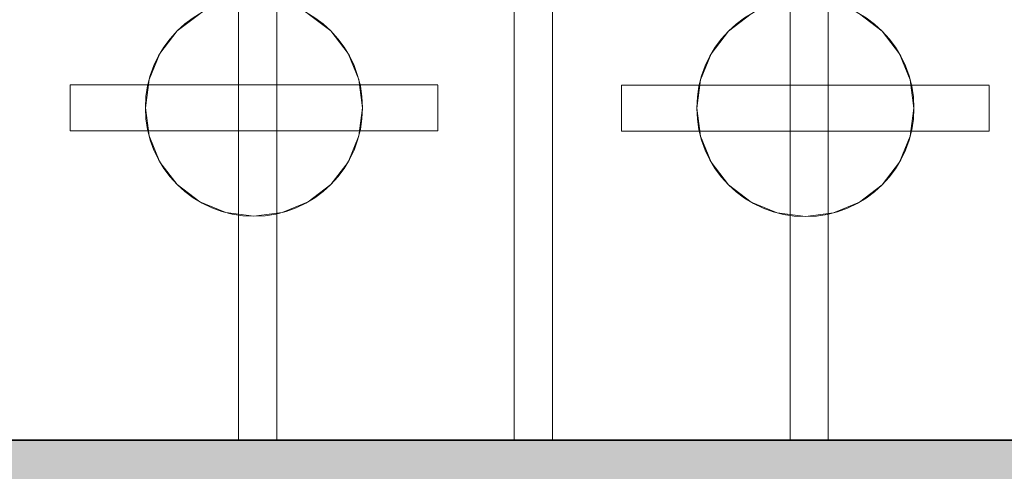
# Model space of a CAD drawing. Units: inches. Extents: x 2696 to 3240, y 1564 to 2310.
# Tile 69 of 76: x 3144.264 to 3152.299, y 2074.447 to 2078.132. Entities that reach past the tile are written whole.
import ezdxf

# ---------------------------------------------------------------- set-up
doc = ezdxf.new("R2010")
doc.units = ezdxf.units.IN
for name, color, linetype, lineweight in [('A-ANNO-DIMS', 3, 'Continuous', 18), ('A-FLOR-FIXT', 8, 'Continuous', 18), ('A-FURN', 251, 'Continuous', 13), ('A-WALL', 7, 'Continuous', 35), ('A-WALL-PATT', 9, 'Continuous', 13)]:
    doc.layers.add(name, color=color, linetype=linetype, lineweight=lineweight)
doc.layers.add('FURNITURE', color=250, linetype='Continuous')
doc.styles.add('TIMES NEW', font='times.ttf')
doc.dimstyles.new('Siddhuu', dxfattribs={"dimtxt": 6, "dimasz": 2.5, "dimexe": 1.25, "dimexo": 0.625, "dimtad": 1, "dimdec": 1, "dimlunit": 4, "dimtxsty": 'TIMES NEW', "dimcen": 2.5, "dimclrd": 256, "dimclre": 1, "dimclrt": 7, "dimadec": 0, "dimazin": 0, "dimtfac": 1, "dimtdec": 1, "dimtmove": 0, "dimatfit": 3, "dimfxl": 1, "dimtolj": 1, "dimlwd": -1, "dimarcsym": 0})

# ---------------------------------------------------------------- blocks, each defined once
blk = doc.blocks.new('A$C1af1f523')
at = {"layer": 'A-FURN'}
for p, q in [((-2.9003, 3.9351), (-2.9003, 0.9365)), ((-2.9003, 3.9351, 0.5), (-2.9003, 0.9365, 0.5)), ((-2.9003, 3.9351), (-2.9003, 3.9351, 0.5)), ((-2.5253, 3.9351), (-2.9003, 3.9351)), ((-2.5253, 3.9351, 0.5), (-2.9003, 3.9351, 0.5)), ((-2.5253, 3.9351), (-2.5253, 0.9365)), ((-2.5253, 3.9351, 0.5), (-2.5253, 0.9365, 0.5)), ((-2.5253, 3.9351), (-2.5253, 3.9351, 0.5)), ((-2.7128, 3.3215), (-2.7128, 3.3215, 0.5)), ((-2.9421, 3.2913), (-2.9421, 3.2913, 0.5)), ((-2.4835, 3.2913), (-2.4835, 3.2913, 0.5)), ((-3.1558, 3.2028), (-3.1558, 3.2028, 0.5)), ((-2.2698, 3.2028), (-2.2698, 3.2028, 0.5)), ((-3.3393, 3.062), (-3.3393, 3.062, 0.5)), ((-2.0863, 3.062), (-2.0863, 3.062, 0.5)), ((-1.9455, 2.8785), (-1.9455, 2.8785, 0.5)), ((-1.857, 2.6648), (-1.857, 2.6648, 0.5)), ((0, 2.5605), (-4.2116, 2.5605)), ((0, 2.5605, 0.5), (-4.2116, 2.5605, 0.5)), ((-1.8268, 2.4355), (-1.8268, 2.4355, 0.5)), ((0, 2.248), (-4.2116, 2.248)), ((0, 2.248, 0.5), (-4.2116, 2.248, 0.5)), ((-1.857, 2.2061), (-1.857, 2.2061, 0.5)), ((-1.9455, 1.9924), (-1.9455, 1.9924, 0.5)), ((-3.3393, 1.8089), (-3.3393, 1.8089, 0.5)), ((-2.0863, 1.8089), (-2.0863, 1.8089, 0.5)), ((-3.1558, 1.6681), (-3.1558, 1.6681, 0.5)), ((-2.2698, 1.6681), (-2.2698, 1.6681, 0.5)), ((-2.9421, 1.5796), (-2.9421, 1.5796, 0.5)), ((-2.7128, 1.5494), (-2.7128, 1.5494, 0.5)), ((-2.4835, 1.5796), (-2.4835, 1.5796, 0.5)), ((-2.9003, 0.9365), (-2.9003, 0.9365, 0.5)), ((-2.5253, 0.9365), (-2.8979, 0.9365)), ((-2.5253, 0.9365, 0.5), (-2.8979, 0.9365, 0.5)), ((-2.8979, 0.9365), (-2.8979, 0.9365, 0.5)), ((-2.5253, 0.9365), (-2.5253, 0.9365, 0.5)), ((0, 0.3125), (-6.5015, 0.3125)), ((0, 0.3125, 0.5), (-6.5015, 0.3125, 0.5)), ((0, 0), (-6.5015, 0)), ((0, 0, 0.5), (-6.5015, 0, 0.5)), ((-2.898, -0.5642), (-2.898, -3.5628)), ((-2.898, -0.5642, 0.5), (-2.898, -3.5628, 0.5)), ((-2.898, -0.5642), (-2.898, -0.5642, 0.5)), ((-2.523, -0.5642), (-2.898, -0.5642)), ((-2.523, -0.5642, 0.5), (-2.898, -0.5642, 0.5)), ((-2.523, -0.5642), (-2.523, -3.5628)), ((-2.523, -0.5642, 0.5), (-2.523, -3.5628, 0.5)), ((-2.523, -0.5642), (-2.523, -0.5642, 0.5)), ((-2.7105, -1.1778), (-2.7105, -1.1778, 0.5)), ((-2.9398, -1.208), (-2.9398, -1.208, 0.5)), ((-2.4812, -1.208), (-2.4812, -1.208, 0.5)), ((-3.1535, -1.2965), (-3.1535, -1.2965, 0.5)), ((-2.2675, -1.2965), (-2.2675, -1.2965, 0.5)), ((-3.337, -1.4373), (-3.337, -1.4373, 0.5)), ((-2.084, -1.4373), (-2.084, -1.4373, 0.5)), ((-1.9432, -1.6208), (-1.9432, -1.6208, 0.5)), ((-1.8547, -1.8345), (-1.8547, -1.8345, 0.5)), ((0, -1.9388), (-4.2094, -1.9388)), ((0, -1.9388, 0.5), (-4.2094, -1.9388, 0.5)), ((-1.8245, -2.0638), (-1.8245, -2.0638, 0.5)), ((0, -2.2513), (-4.2094, -2.2513)), ((0, -2.2513, 0.5), (-4.2094, -2.2513, 0.5)), ((-1.8547, -2.2931), (-1.8547, -2.2931, 0.5)), ((-1.9432, -2.5068), (-1.9432, -2.5068, 0.5)), ((-3.337, -2.6903), (-3.337, -2.6903, 0.5)), ((-2.084, -2.6903), (-2.084, -2.6903, 0.5)), ((-3.1535, -2.8311), (-3.1535, -2.8311, 0.5)), ((-2.2675, -2.8311), (-2.2675, -2.8311, 0.5)), ((-2.9398, -2.9196), (-2.9398, -2.9196, 0.5)), ((-2.7105, -2.9498), (-2.7105, -2.9498, 0.5)), ((-2.4812, -2.9196), (-2.4812, -2.9196, 0.5)), ((-2.898, -3.5628), (-2.898, -3.5628, 0.5)), ((-2.523, -3.5628), (-2.8956, -3.5628)), ((-2.523, -3.5628, 0.5), (-2.8956, -3.5628, 0.5)), ((-2.8956, -3.5628), (-2.8956, -3.5628, 0.5)), ((-2.523, -3.5628), (-2.523, -3.5628, 0.5))]:
    blk.add_line(p, q, dxfattribs=at)
for centre in [(-2.7128, 2.4355), (-2.7128, 2.4355, 0.5), (-2.7105, -2.0638), (-2.7105, -2.0638, 0.5)]:
    blk.add_circle(centre, 0.886, dxfattribs=at)
at = {"layer": 'FURNITURE'}
for p, q in [((0, 2.5605), (0, 2.5605, 0.5)), ((0, 2.248), (0, 2.248, 0.5)), ((0, 0.3125), (0, 0.3125, 0.5)), ((0, 0), (0, 0, 0.5)), ((0, -1.9388), (0, -1.9388, 0.5)), ((0, -2.2513), (0, -2.2513, 0.5))]:
    blk.add_line(p, q, dxfattribs=at)
at = {"layer": 'A-FURN'}
mesh = blk.add_polyface(dxfattribs=at)
corners = [(-2.9003, 0.9365, 0.5), (-2.9003, 3.9351), (-2.9003, 0.9365), (-2.9003, 3.9351, 0.5)]
mesh.append_faces([[corners[k] for k in face] for face in [(2, 1, 0), (3, 0, 1)]], dxfattribs={"vtx1": -1})
mesh = blk.add_polyface(dxfattribs=at)
corners = [(-2.5253, 3.9351, 0.5), (-2.9003, 3.9351), (-2.9003, 3.9351, 0.5), (-2.5253, 3.9351)]
mesh.append_faces([[corners[k] for k in face] for face in [(2, 1, 0), (3, 0, 1)]], dxfattribs={"vtx1": -1})
mesh = blk.add_polyface(dxfattribs=at)
corners = [(-2.5253, 0.9365, 0.5), (-2.5253, 3.9351), (-2.5253, 0.9365), (-2.5253, 3.9351, 0.5)]
mesh.append_faces([[corners[k] for k in face] for face in [(2, 1, 0), (3, 0, 1)]], dxfattribs={"vtx1": -1})
mesh = blk.add_polyface(dxfattribs=at)
corners = [(-2.7128, 3.3215), (-2.9421, 3.2913, 0.5), (-2.9421, 3.2913), (-2.7128, 3.3215, 0.5)]
mesh.append_faces([[corners[k] for k in face] for face in [(2, 1, 0), (3, 0, 1)]], dxfattribs={"vtx1": -1})
mesh = blk.add_polyface(dxfattribs=at)
corners = [(-2.4835, 3.2913), (-2.7128, 3.3215, 0.5), (-2.7128, 3.3215), (-2.4835, 3.2913, 0.5)]
mesh.append_faces([[corners[k] for k in face] for face in [(2, 1, 0), (3, 0, 1)]], dxfattribs={"vtx1": -1})
mesh = blk.add_polyface(dxfattribs=at)
corners = [(-2.9421, 3.2913), (-3.1558, 3.2028, 0.5), (-3.1558, 3.2028), (-2.9421, 3.2913, 0.5)]
mesh.append_faces([[corners[k] for k in face] for face in [(2, 1, 0), (3, 0, 1)]], dxfattribs={"vtx1": -1})
mesh = blk.add_polyface(dxfattribs=at)
corners = [(-2.2698, 3.2028), (-2.4835, 3.2913, 0.5), (-2.4835, 3.2913), (-2.2698, 3.2028, 0.5)]
mesh.append_faces([[corners[k] for k in face] for face in [(2, 1, 0), (3, 0, 1)]], dxfattribs={"vtx1": -1})
mesh = blk.add_polyface(dxfattribs=at)
corners = [(-3.1558, 3.2028), (-3.3393, 3.062, 0.5), (-3.3393, 3.062), (-3.1558, 3.2028, 0.5)]
mesh.append_faces([[corners[k] for k in face] for face in [(2, 1, 0), (3, 0, 1)]], dxfattribs={"vtx1": -1})
mesh = blk.add_polyface(dxfattribs=at)
corners = [(-2.0863, 3.062), (-2.2698, 3.2028, 0.5), (-2.2698, 3.2028), (-2.0863, 3.062, 0.5)]
mesh.append_faces([[corners[k] for k in face] for face in [(2, 1, 0), (3, 0, 1)]], dxfattribs={"vtx1": -1})
mesh = blk.add_polyface(dxfattribs=at)
corners = [(-3.3393, 3.062, 0.5), (-3.4801, 2.8785), (-3.3393, 3.062), (-3.4801, 2.8785, 0.5)]
mesh.append_faces([[corners[k] for k in face] for face in [(2, 1, 0), (3, 0, 1)]], dxfattribs={"vtx1": -1})
mesh = blk.add_polyface(dxfattribs=at)
corners = [(-1.9455, 2.8785, 0.5), (-2.0863, 3.062), (-1.9455, 2.8785), (-2.0863, 3.062, 0.5)]
mesh.append_faces([[corners[k] for k in face] for face in [(2, 1, 0), (3, 0, 1)]], dxfattribs={"vtx1": -1})
mesh = blk.add_polyface(dxfattribs=at)
corners = [(-1.857, 2.6648, 0.5), (-1.9455, 2.8785), (-1.857, 2.6648), (-1.9455, 2.8785, 0.5)]
mesh.append_faces([[corners[k] for k in face] for face in [(2, 1, 0), (3, 0, 1)]], dxfattribs={"vtx1": -1})
mesh = blk.add_polyface(dxfattribs=at)
corners = [(-1.8268, 2.4355, 0.5), (-1.857, 2.6648), (-1.8268, 2.4355), (-1.857, 2.6648, 0.5)]
mesh.append_faces([[corners[k] for k in face] for face in [(2, 1, 0), (3, 0, 1)]], dxfattribs={"vtx1": -1})
mesh = blk.add_polyface(dxfattribs=at)
corners = [(0, 2.5605, 0.5), (-4.2116, 2.5605), (-4.2116, 2.5605, 0.5), (0, 2.5605)]
mesh.append_faces([[corners[k] for k in face] for face in [(2, 1, 0), (3, 0, 1)]], dxfattribs={"vtx1": -1})
mesh = blk.add_polyface(dxfattribs=at)
corners = [(-1.857, 2.2061, 0.5), (-1.8268, 2.4355), (-1.857, 2.2061), (-1.8268, 2.4355, 0.5)]
mesh.append_faces([[corners[k] for k in face] for face in [(2, 1, 0), (3, 0, 1)]], dxfattribs={"vtx1": -1})
mesh = blk.add_polyface(dxfattribs=at)
corners = [(0, 2.248, 0.5), (-4.2116, 2.248), (-4.2116, 2.248, 0.5), (0, 2.248)]
mesh.append_faces([[corners[k] for k in face] for face in [(2, 1, 0), (3, 0, 1)]], dxfattribs={"vtx1": -1})
mesh = blk.add_polyface(dxfattribs=at)
corners = [(-1.9455, 1.9924, 0.5), (-1.857, 2.2061), (-1.9455, 1.9924), (-1.857, 2.2061, 0.5)]
mesh.append_faces([[corners[k] for k in face] for face in [(2, 1, 0), (3, 0, 1)]], dxfattribs={"vtx1": -1})
mesh = blk.add_polyface(dxfattribs=at)
corners = [(-3.4801, 1.9924, 0.5), (-3.3393, 1.8089), (-3.4801, 1.9924), (-3.3393, 1.8089, 0.5)]
mesh.append_faces([[corners[k] for k in face] for face in [(2, 1, 0), (3, 0, 1)]], dxfattribs={"vtx1": -1})
mesh = blk.add_polyface(dxfattribs=at)
corners = [(-2.0863, 1.8089, 0.5), (-1.9455, 1.9924), (-2.0863, 1.8089), (-1.9455, 1.9924, 0.5)]
mesh.append_faces([[corners[k] for k in face] for face in [(2, 1, 0), (3, 0, 1)]], dxfattribs={"vtx1": -1})
mesh = blk.add_polyface(dxfattribs=at)
corners = [(-3.1558, 1.6681, 0.5), (-3.3393, 1.8089), (-3.3393, 1.8089, 0.5), (-3.1558, 1.6681)]
mesh.append_faces([[corners[k] for k in face] for face in [(2, 1, 0), (3, 0, 1)]], dxfattribs={"vtx1": -1})
mesh = blk.add_polyface(dxfattribs=at)
corners = [(-2.0863, 1.8089, 0.5), (-2.2698, 1.6681), (-2.2698, 1.6681, 0.5), (-2.0863, 1.8089)]
mesh.append_faces([[corners[k] for k in face] for face in [(2, 1, 0), (3, 0, 1)]], dxfattribs={"vtx1": -1})
mesh = blk.add_polyface(dxfattribs=at)
corners = [(-2.9421, 1.5796, 0.5), (-3.1558, 1.6681), (-3.1558, 1.6681, 0.5), (-2.9421, 1.5796)]
mesh.append_faces([[corners[k] for k in face] for face in [(2, 1, 0), (3, 0, 1)]], dxfattribs={"vtx1": -1})
mesh = blk.add_polyface(dxfattribs=at)
corners = [(-2.2698, 1.6681, 0.5), (-2.4835, 1.5796), (-2.4835, 1.5796, 0.5), (-2.2698, 1.6681)]
mesh.append_faces([[corners[k] for k in face] for face in [(2, 1, 0), (3, 0, 1)]], dxfattribs={"vtx1": -1})
mesh = blk.add_polyface(dxfattribs=at)
corners = [(-2.7128, 1.5494, 0.5), (-2.9421, 1.5796), (-2.9421, 1.5796, 0.5), (-2.7128, 1.5494)]
mesh.append_faces([[corners[k] for k in face] for face in [(2, 1, 0), (3, 0, 1)]], dxfattribs={"vtx1": -1})
mesh = blk.add_polyface(dxfattribs=at)
corners = [(-2.4835, 1.5796, 0.5), (-2.7128, 1.5494), (-2.7128, 1.5494, 0.5), (-2.4835, 1.5796)]
mesh.append_faces([[corners[k] for k in face] for face in [(2, 1, 0), (3, 0, 1)]], dxfattribs={"vtx1": -1})
mesh = blk.add_polyface(dxfattribs=at)
corners = [(-2.5253, 0.9365, 0.5), (-2.8979, 0.9365), (-2.8979, 0.9365, 0.5), (-2.5253, 0.9365)]
mesh.append_faces([[corners[k] for k in face] for face in [(2, 1, 0), (3, 0, 1)]], dxfattribs={"vtx1": -1})
mesh = blk.add_polyface(dxfattribs=at)
corners = [(0, 0.3125, 0.5), (-6.5015, 0.3125), (-6.5015, 0.3125, 0.5), (0, 0.3125)]
mesh.append_faces([[corners[k] for k in face] for face in [(2, 1, 0), (3, 0, 1)]], dxfattribs={"vtx1": -1})
mesh = blk.add_polyface(dxfattribs=at)
corners = [(0, 0, 0.5), (-6.5015, 0), (-6.5015, 0, 0.5), (0, 0)]
mesh.append_faces([[corners[k] for k in face] for face in [(2, 1, 0), (3, 0, 1)]], dxfattribs={"vtx1": -1})
mesh = blk.add_polyface(dxfattribs=at)
corners = [(-2.898, -3.5628, 0.5), (-2.898, -0.5642), (-2.898, -3.5628), (-2.898, -0.5642, 0.5)]
mesh.append_faces([[corners[k] for k in face] for face in [(2, 1, 0), (3, 0, 1)]], dxfattribs={"vtx1": -1})
mesh = blk.add_polyface(dxfattribs=at)
corners = [(-2.523, -0.5642, 0.5), (-2.898, -0.5642), (-2.898, -0.5642, 0.5), (-2.523, -0.5642)]
mesh.append_faces([[corners[k] for k in face] for face in [(2, 1, 0), (3, 0, 1)]], dxfattribs={"vtx1": -1})
mesh = blk.add_polyface(dxfattribs=at)
corners = [(-2.523, -3.5628, 0.5), (-2.523, -0.5642), (-2.523, -3.5628), (-2.523, -0.5642, 0.5)]
mesh.append_faces([[corners[k] for k in face] for face in [(2, 1, 0), (3, 0, 1)]], dxfattribs={"vtx1": -1})
mesh = blk.add_polyface(dxfattribs=at)
corners = [(-2.7105, -1.1778), (-2.9398, -1.208, 0.5), (-2.9398, -1.208), (-2.7105, -1.1778, 0.5)]
mesh.append_faces([[corners[k] for k in face] for face in [(2, 1, 0), (3, 0, 1)]], dxfattribs={"vtx1": -1})
mesh = blk.add_polyface(dxfattribs=at)
corners = [(-2.4812, -1.208), (-2.7105, -1.1778, 0.5), (-2.7105, -1.1778), (-2.4812, -1.208, 0.5)]
mesh.append_faces([[corners[k] for k in face] for face in [(2, 1, 0), (3, 0, 1)]], dxfattribs={"vtx1": -1})
mesh = blk.add_polyface(dxfattribs=at)
corners = [(-2.9398, -1.208), (-3.1535, -1.2965, 0.5), (-3.1535, -1.2965), (-2.9398, -1.208, 0.5)]
mesh.append_faces([[corners[k] for k in face] for face in [(2, 1, 0), (3, 0, 1)]], dxfattribs={"vtx1": -1})
mesh = blk.add_polyface(dxfattribs=at)
corners = [(-2.2675, -1.2965), (-2.4812, -1.208, 0.5), (-2.4812, -1.208), (-2.2675, -1.2965, 0.5)]
mesh.append_faces([[corners[k] for k in face] for face in [(2, 1, 0), (3, 0, 1)]], dxfattribs={"vtx1": -1})
mesh = blk.add_polyface(dxfattribs=at)
corners = [(-3.1535, -1.2965), (-3.337, -1.4373, 0.5), (-3.337, -1.4373), (-3.1535, -1.2965, 0.5)]
mesh.append_faces([[corners[k] for k in face] for face in [(2, 1, 0), (3, 0, 1)]], dxfattribs={"vtx1": -1})
mesh = blk.add_polyface(dxfattribs=at)
corners = [(-2.084, -1.4373), (-2.2675, -1.2965, 0.5), (-2.2675, -1.2965), (-2.084, -1.4373, 0.5)]
mesh.append_faces([[corners[k] for k in face] for face in [(2, 1, 0), (3, 0, 1)]], dxfattribs={"vtx1": -1})
mesh = blk.add_polyface(dxfattribs=at)
corners = [(-3.337, -1.4373, 0.5), (-3.4778, -1.6208), (-3.337, -1.4373), (-3.4778, -1.6208, 0.5)]
mesh.append_faces([[corners[k] for k in face] for face in [(2, 1, 0), (3, 0, 1)]], dxfattribs={"vtx1": -1})
mesh = blk.add_polyface(dxfattribs=at)
corners = [(-1.9432, -1.6208, 0.5), (-2.084, -1.4373), (-1.9432, -1.6208), (-2.084, -1.4373, 0.5)]
mesh.append_faces([[corners[k] for k in face] for face in [(2, 1, 0), (3, 0, 1)]], dxfattribs={"vtx1": -1})
mesh = blk.add_polyface(dxfattribs=at)
corners = [(-1.8547, -1.8345, 0.5), (-1.9432, -1.6208), (-1.8547, -1.8345), (-1.9432, -1.6208, 0.5)]
mesh.append_faces([[corners[k] for k in face] for face in [(2, 1, 0), (3, 0, 1)]], dxfattribs={"vtx1": -1})
mesh = blk.add_polyface(dxfattribs=at)
corners = [(-1.8245, -2.0638, 0.5), (-1.8547, -1.8345), (-1.8245, -2.0638), (-1.8547, -1.8345, 0.5)]
mesh.append_faces([[corners[k] for k in face] for face in [(2, 1, 0), (3, 0, 1)]], dxfattribs={"vtx1": -1})
mesh = blk.add_polyface(dxfattribs=at)
corners = [(0, -1.9388, 0.5), (-4.2094, -1.9388), (-4.2094, -1.9388, 0.5), (0, -1.9388)]
mesh.append_faces([[corners[k] for k in face] for face in [(2, 1, 0), (3, 0, 1)]], dxfattribs={"vtx1": -1})
mesh = blk.add_polyface(dxfattribs=at)
corners = [(-1.8547, -2.2931, 0.5), (-1.8245, -2.0638), (-1.8547, -2.2931), (-1.8245, -2.0638, 0.5)]
mesh.append_faces([[corners[k] for k in face] for face in [(2, 1, 0), (3, 0, 1)]], dxfattribs={"vtx1": -1})
mesh = blk.add_polyface(dxfattribs=at)
corners = [(0, -2.2513, 0.5), (-4.2094, -2.2513), (-4.2094, -2.2513, 0.5), (0, -2.2513)]
mesh.append_faces([[corners[k] for k in face] for face in [(2, 1, 0), (3, 0, 1)]], dxfattribs={"vtx1": -1})
mesh = blk.add_polyface(dxfattribs=at)
corners = [(-1.9432, -2.5068, 0.5), (-1.8547, -2.2931), (-1.9432, -2.5068), (-1.8547, -2.2931, 0.5)]
mesh.append_faces([[corners[k] for k in face] for face in [(2, 1, 0), (3, 0, 1)]], dxfattribs={"vtx1": -1})
mesh = blk.add_polyface(dxfattribs=at)
corners = [(-3.4778, -2.5068, 0.5), (-3.337, -2.6903), (-3.4778, -2.5068), (-3.337, -2.6903, 0.5)]
mesh.append_faces([[corners[k] for k in face] for face in [(2, 1, 0), (3, 0, 1)]], dxfattribs={"vtx1": -1})
mesh = blk.add_polyface(dxfattribs=at)
corners = [(-2.084, -2.6903, 0.5), (-1.9432, -2.5068), (-2.084, -2.6903), (-1.9432, -2.5068, 0.5)]
mesh.append_faces([[corners[k] for k in face] for face in [(2, 1, 0), (3, 0, 1)]], dxfattribs={"vtx1": -1})
mesh = blk.add_polyface(dxfattribs=at)
corners = [(-3.1535, -2.8311, 0.5), (-3.337, -2.6903), (-3.337, -2.6903, 0.5), (-3.1535, -2.8311)]
mesh.append_faces([[corners[k] for k in face] for face in [(2, 1, 0), (3, 0, 1)]], dxfattribs={"vtx1": -1})
mesh = blk.add_polyface(dxfattribs=at)
corners = [(-2.084, -2.6903, 0.5), (-2.2675, -2.8311), (-2.2675, -2.8311, 0.5), (-2.084, -2.6903)]
mesh.append_faces([[corners[k] for k in face] for face in [(2, 1, 0), (3, 0, 1)]], dxfattribs={"vtx1": -1})
mesh = blk.add_polyface(dxfattribs=at)
corners = [(-2.9398, -2.9196, 0.5), (-3.1535, -2.8311), (-3.1535, -2.8311, 0.5), (-2.9398, -2.9196)]
mesh.append_faces([[corners[k] for k in face] for face in [(2, 1, 0), (3, 0, 1)]], dxfattribs={"vtx1": -1})
mesh = blk.add_polyface(dxfattribs=at)
corners = [(-2.2675, -2.8311, 0.5), (-2.4812, -2.9196), (-2.4812, -2.9196, 0.5), (-2.2675, -2.8311)]
mesh.append_faces([[corners[k] for k in face] for face in [(2, 1, 0), (3, 0, 1)]], dxfattribs={"vtx1": -1})
mesh = blk.add_polyface(dxfattribs=at)
corners = [(-2.7105, -2.9498, 0.5), (-2.9398, -2.9196), (-2.9398, -2.9196, 0.5), (-2.7105, -2.9498)]
mesh.append_faces([[corners[k] for k in face] for face in [(2, 1, 0), (3, 0, 1)]], dxfattribs={"vtx1": -1})
mesh = blk.add_polyface(dxfattribs=at)
corners = [(-2.4812, -2.9196, 0.5), (-2.7105, -2.9498), (-2.7105, -2.9498, 0.5), (-2.4812, -2.9196)]
mesh.append_faces([[corners[k] for k in face] for face in [(2, 1, 0), (3, 0, 1)]], dxfattribs={"vtx1": -1})
mesh = blk.add_polyface(dxfattribs=at)
corners = [(-2.523, -3.5628, 0.5), (-2.8956, -3.5628), (-2.8956, -3.5628, 0.5), (-2.523, -3.5628)]
mesh.append_faces([[corners[k] for k in face] for face in [(2, 1, 0), (3, 0, 1)]], dxfattribs={"vtx1": -1})
blk = doc.blocks.new('*D54')
at = {"layer": 'A-ANNO-DIMS', "color": 1, "lineweight": -2, "transparency": 16777216}
for p, q in [((3124.6114, 1893.8261), (3124.6114, 2298.4511)), ((3136.6114, 1893.8261), (3136.6114, 2298.4511))]:
    blk.add_line(p, q, dxfattribs=at)
at = {"layer": 'A-ANNO-DIMS', "transparency": 16777216}
for p, q in [((3127.1114, 2297.2011), (3134.1114, 2297.2011)), ((3136.6114, 2297.2011), (3155.7572, 2297.2011))]:
    blk.add_line(p, q, dxfattribs=at)
for points in [[(3127.1114, 2297.6178), (3127.1114, 2296.7844), (3124.6114, 2297.2011)], [(3134.1114, 2297.6178), (3134.1114, 2296.7844), (3136.6114, 2297.2011)]]:
    blk.add_solid(points, dxfattribs=at)
at = {"layer": 'Defpoints', "color": 0, "transparency": 16777216}
for p in [(3136.6114, 2297.2011), (3124.6114, 1893.2011), (3136.6114, 1893.2011)]:
    blk.add_point(p, dxfattribs=at)
at = {"layer": 'A-ANNO-DIMS', "color": 7, "transparency": 16777216, "insert": (3147.4343, 2300.878), "char_height": 6, "attachment_point": 5, "style": 'TIMES NEW'}
blk.add_mtext('\\A1;1\'-0"', dxfattribs=at)

msp = doc.modelspace()

# ---------------------------------------------------------------- hatches: boundary and pattern name
at = {"layer": 'A-WALL-PATT', "transparency": 33554556}
h = msp.add_hatch(color=256, dxfattribs=at)
h.dxf.hatch_style = 1
h.paths.add_polyline_path([(2879.1114, 2253.2011), (2905.9101, 2253.2011), (2905.9101, 2262.2011), (2841.889, 2262.2011), (2841.889, 2253.2011), (2870.1114, 2253.2011), (2870.1114, 2176.6011), (2965.7088, 2176.6011), (2965.7088, 2206.7011), (2973.5828, 2206.7011), (2973.5828, 2215.7011), (2965.7088, 2215.7011), (2965.7088, 2262.2011), (2929.9101, 2262.2011), (2929.9101, 2253.2011), (2956.7088, 2253.2011), (2956.7088, 2185.6011), (2879.1114, 2185.6011)])
h.paths.add_polyline_path([(2782.8338, 2262.2011), (2745.6114, 2262.2011), (2745.6114, 2228.7287), (2754.6114, 2228.7287), (2754.6114, 2253.2011), (2782.8338, 2253.2011)])
h.paths.add_polyline_path([(2754.6114, 2136.2011), (2965.7088, 2136.2011), (2965.7088, 2145.2011), (2879.1114, 2145.2011), (2879.1114, 2147.0735), (2877.3397, 2147.0735), (2870.1114, 2147.0735), (2870.1114, 2145.2011), (2754.6114, 2145.2011), (2754.6114, 2169.6735), (2745.6114, 2169.6735), (2745.6114, 2000.2011), (2754.6114, 2000.2011), (2754.6114, 2019.2011), (2849.0828, 2019.2011), (2849.0828, 2023.7011), (2841.2088, 2023.7011), (2841.2088, 2051.8271), (2836.7088, 2051.8271), (2836.7088, 2023.7011), (2754.6114, 2023.7011), (2754.6114, 2091.2011), (2836.7088, 2091.2011), (2836.7088, 2087.8271), (2841.2088, 2087.8271), (2841.2088, 2095.7011), (2754.6114, 2095.7011)])
h.paths.add_polyline_path([(2965.7088, 2136.2011), (2956.7088, 2136.2011), (2956.7088, 2023.7011), (2885.0828, 2023.7011), (2885.0828, 2019.2011), (2956.7088, 2019.2011), (2956.7088, 1950.5751), (2965.7088, 1950.5751), (2965.7088, 1980.2011), (2973.5828, 1980.2011), (2973.5828, 1989.2011), (2965.7088, 1989.2011)])
h.paths.add_polyline_path([(2754.6114, 1906.7011), (2880.2088, 1906.7011), (2884.7088, 1906.7011), (2956.7088, 1906.7011), (2956.7088, 1792.7011), (2944.7088, 1792.7011), (2944.7088, 1783.7011), (2956.7088, 1783.7011), (2956.7088, 1740.2011), (2884.7088, 1740.2011), (2884.7088, 1783.7011), (2896.7088, 1783.7011), (2896.7088, 1792.7011), (2884.7088, 1792.7011), (2884.7088, 1846.7011), (2880.2088, 1846.7011), (2880.2088, 1740.2011), (2754.6114, 1740.2011), (2754.6114, 1777.2011), (2745.6114, 1777.2011), (2745.6114, 1692.7011), (2754.6114, 1692.7011), (2754.6114, 1731.2011), (2956.7088, 1731.2011), (2956.7088, 1723.3271), (2965.7088, 1723.3271), (2965.7088, 1884.2011), (2973.5828, 1884.2011), (2973.5828, 1893.2011), (2965.7088, 1893.2011), (2965.7088, 1914.5751), (2956.7088, 1914.5751), (2956.7088, 1911.2011), (2754.6114, 1911.2011), (2754.6114, 1930.2011), (2745.6114, 1930.2011), (2745.6114, 1817.2011), (2754.6114, 1817.2011), (2754.6114, 1854.2011), (2826.6114, 1854.2011), (2826.6114, 1868.8271), (2822.1114, 1868.8271), (2822.1114, 1858.7011), (2754.6114, 1858.7011)])
h.paths.add_polyline_path([(2965.7088, 1656.2011), (3008.2374, 1656.2011), (3008.2374, 1665.2011), (2965.7088, 1665.2011), (2965.7088, 1693.3271), (2956.7088, 1693.3271), (2956.7088, 1686.2011), (2934.5828, 1686.2011), (2934.5828, 1681.7011), (2956.7088, 1681.7011), (2956.7088, 1614.2011), (2896.7088, 1614.2011), (2896.7088, 1681.7011), (2904.5828, 1681.7011), (2904.5828, 1686.2011), (2892.2088, 1686.2011), (2892.2088, 1614.2011), (2858.4101, 1614.2011), (2858.4101, 1605.2011), (2965.7088, 1605.2011)])
h.paths.add_polyline_path([(2788.4101, 1614.2011), (2754.6114, 1614.2011), (2754.6114, 1652.7011), (2745.6114, 1652.7011), (2745.6114, 1605.2011), (2788.4101, 1605.2011)])
h.paths.add_polyline_path([(3199.6114, 1633.0476), (3190.6114, 1633.0476), (3190.6114, 1614.2011), (3082.6114, 1614.2011), (3082.6114, 1665.2011), (3070.2374, 1665.2011), (3070.2374, 1656.2011), (3078.1114, 1656.2011), (3078.1114, 1605.2011), (3199.6114, 1605.2011)])
h.paths.add_polyline_path([(3199.6114, 1702.0476), (3190.6114, 1702.0476), (3190.6114, 1699.7011), (3106.6114, 1699.7011), (3106.6114, 1747.7011), (3190.6114, 1747.7011), (3190.6114, 1752.2011), (3082.6114, 1752.2011), (3082.6114, 1760.0751), (3078.1114, 1760.0751), (3078.1114, 1747.7011), (3102.1114, 1747.7011), (3102.1114, 1699.7011), (3078.1114, 1699.7011), (3078.1114, 1695.2011), (3190.6114, 1695.2011), (3190.6114, 1676.3546), (3199.6114, 1676.3546)])
h.paths.add_polyline_path([(3199.6114, 1783.2011), (3190.6114, 1783.2011), (3190.6114, 1745.3546), (3199.6114, 1745.3546)])
h.paths.add_polyline_path([(3082.6114, 1884.2011), (3190.6114, 1884.2011), (3190.6114, 1853.2011), (3199.6114, 1853.2011), (3199.6114, 1901.7011), (3190.6114, 1901.7011), (3190.6114, 1893.2011), (3005.5828, 1893.2011), (3005.5828, 1891.2811), (3005.5828, 1884.2011), (3078.1114, 1884.2011), (3078.1114, 1792.0751), (3082.6114, 1792.0751)])
h.paths.add_polyline_path([(3199.6114, 1994.7011), (3190.6114, 1994.7011), (3190.6114, 1989.2011), (3073.7088, 1989.2011), (3073.7088, 2034.2011), (3069.2088, 2034.2011), (3069.2088, 1989.2011), (3005.5828, 1989.2011), (3005.5828, 1980.2011), (3190.6114, 1980.2011), (3190.6114, 1971.7011), (3199.6114, 1971.7011)])
h.paths.add_polyline_path([(3199.6114, 2155.2011), (3190.6114, 2155.2011), (3190.6114, 2064.7011), (3199.6114, 2064.7011)])
h.paths.add_polyline_path([(3190.6114, 2074.7011), (3106.6114, 2074.7011), (3106.6114, 2122.7011), (3190.6114, 2122.7011), (3190.6114, 2127.2011), (3082.7088, 2127.2011), (3082.7088, 2135.0751), (3073.7088, 2135.0751), (3073.7088, 2122.7011), (3102.1114, 2122.7011), (3102.1114, 2074.7011), (3069.2088, 2074.7011), (3069.2088, 2070.2011), (3190.6114, 2070.2011)])
h.paths.add_polyline_path([(3082.7088, 2253.2011), (3190.6114, 2253.2011), (3190.6114, 2225.2011), (3199.6114, 2225.2011), (3199.6114, 2262.2011), (3073.7088, 2262.2011), (3073.7088, 2215.7011), (3035.5828, 2215.7011), (3035.5828, 2206.7011), (3073.7088, 2206.7011), (3073.7088, 2171.0751), (3082.7088, 2171.0751)])

# ---------------------------------------------------------------- linework, layer by layer
at = {"layer": 'A-WALL'}
msp.add_line((3106.6114, 2074.7011), (3190.6114, 2074.7011), dxfattribs=at)

# ---------------------------------------------------------------- block references
at = {"layer": 'A-FLOR-FIXT', "xscale": -1, "rotation": 90}
msp.add_blockref('A$C1af1f523', (3148.6114, 2074.7011), dxfattribs=at)

# ---------------------------------------------------------------- dimensions: what is measured, and where the dimension line sits
at = {"layer": 'A-ANNO-DIMS'}
dim = msp.add_linear_dim(base=(3136.6114, 2297.2011), p1=(3124.6114, 1893.2011), p2=(3136.6114, 1893.2011), dimstyle='Siddhuu', override={"dimdec": 1, "dimlfac": 1, "dimrnd": 0, "dimzin": 1, "dimdsep": 46, "dimlunit": 4, "dimfrac": 2}, dxfattribs=at)
dim.commit()
dim.dimension.update_dxf_attribs({"geometry": '*D54', "text_midpoint": (3147.4343, 2300.878)})

doc.saveas('drawing.dxf')
